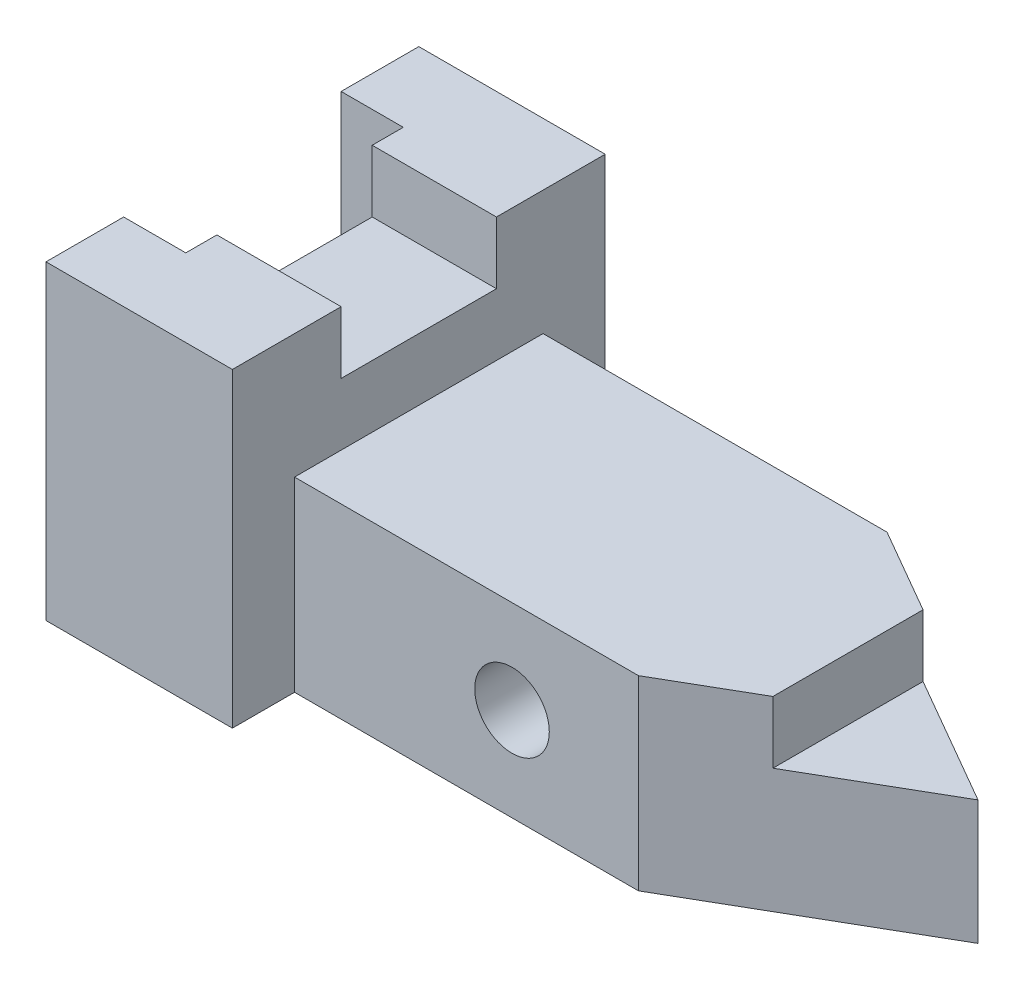
ISO-10303-21;
HEADER;
FILE_DESCRIPTION(('STEP AP214'),'2;1');
FILE_NAME('part.step','',(''),(''),'','','');
FILE_SCHEMA(('AUTOMOTIVE_DESIGN { 1 0 10303 214 1 1 1 1 }'));
ENDSEC;
DATA;
#1=APPLICATION_CONTEXT('core data for automotive mechanical design processes');
#2=APPLICATION_PROTOCOL_DEFINITION('international standard','automotive_design',2000,#1);
#3=PRODUCT_CONTEXT('',#1,'mechanical');
#4=PRODUCT('Part','Part','',(#3));
#5=PRODUCT_RELATED_PRODUCT_CATEGORY('part','',(#4));
#6=PRODUCT_DEFINITION_FORMATION('','',#4);
#7=PRODUCT_DEFINITION_CONTEXT('part definition',#1,'design');
#8=PRODUCT_DEFINITION('design','',#6,#7);
#9=PRODUCT_DEFINITION_SHAPE('','',#8);
#10=(LENGTH_UNIT() NAMED_UNIT(*) SI_UNIT(.MILLI.,.METRE.));
#11=(NAMED_UNIT(*) PLANE_ANGLE_UNIT() SI_UNIT($,.RADIAN.));
#12=(NAMED_UNIT(*) SI_UNIT($,.STERADIAN.) SOLID_ANGLE_UNIT());
#13=UNCERTAINTY_MEASURE_WITH_UNIT(LENGTH_MEASURE(1.E-05),#10,'distance_accuracy_value','');
#14=(GEOMETRIC_REPRESENTATION_CONTEXT(3) GLOBAL_UNCERTAINTY_ASSIGNED_CONTEXT((#13)) GLOBAL_UNIT_ASSIGNED_CONTEXT((#10,
#11,#12)) REPRESENTATION_CONTEXT('',''));
#15=CARTESIAN_POINT('',(0.,0.,0.));
#16=DIRECTION('',(0.,0.,1.));
#17=DIRECTION('',(1.,0.,0.));
#18=AXIS2_PLACEMENT_3D('',#15,#16,#17);
#19=CARTESIAN_POINT('',(0.,0.,30.));
#20=DIRECTION('',(0.,1.,0.));
#21=DIRECTION('',(0.,0.,1.));
#22=AXIS2_PLACEMENT_3D('',#19,#20,#21);
#23=PLANE('',#22);
#24=DIRECTION('',(-1.,0.,0.));
#25=VECTOR('',#24,1.);
#26=CARTESIAN_POINT('',(120.,0.,-20.));
#27=LINE('',#26,#25);
#28=CARTESIAN_POINT('',(85.3589838486219,0.,-20.));
#29=VERTEX_POINT('',#28);
#30=CARTESIAN_POINT('',(30.,0.,-20.));
#31=VERTEX_POINT('',#30);
#32=EDGE_CURVE('E65',#29,#31,#27,.T.);
#33=ORIENTED_EDGE('',*,*,#32,.F.);
#34=DIRECTION('',(-0.866025403784442,0.,-0.499999999999995));
#35=VECTOR('',#34,1.);
#36=CARTESIAN_POINT('',(42.9903810567658,0.,-44.4615242270661));
#37=LINE('',#36,#35);
#38=CARTESIAN_POINT('',(120.,0.,0.));
#39=VERTEX_POINT('',#38);
#40=EDGE_CURVE('E173',#39,#29,#37,.T.);
#41=ORIENTED_EDGE('',*,*,#40,.F.);
#42=DIRECTION('',(-0.866025403784442,0.,0.499999999999995));
#43=VECTOR('',#42,1.);
#44=CARTESIAN_POINT('',(17.0096189432329,0.,59.4615242270658));
#45=LINE('',#44,#43);
#46=CARTESIAN_POINT('',(85.3589838486219,0.,20.));
#47=VERTEX_POINT('',#46);
#48=EDGE_CURVE('E317',#39,#47,#45,.T.);
#49=ORIENTED_EDGE('',*,*,#48,.T.);
#50=DIRECTION('',(-1.,0.,0.));
#51=VECTOR('',#50,1.);
#52=CARTESIAN_POINT('',(120.,0.,20.));
#53=LINE('',#52,#51);
#54=CARTESIAN_POINT('',(30.,0.,20.));
#55=VERTEX_POINT('',#54);
#56=EDGE_CURVE('E194',#47,#55,#53,.T.);
#57=ORIENTED_EDGE('',*,*,#56,.T.);
#58=DIRECTION('',(0.,0.,-1.));
#59=VECTOR('',#58,1.);
#60=CARTESIAN_POINT('',(30.,0.,30.));
#61=LINE('',#60,#59);
#62=CARTESIAN_POINT('',(30.,0.,30.));
#63=VERTEX_POINT('',#62);
#64=EDGE_CURVE('E275',#63,#55,#61,.T.);
#65=ORIENTED_EDGE('',*,*,#64,.F.);
#66=DIRECTION('',(1.,0.,0.));
#67=VECTOR('',#66,1.);
#68=CARTESIAN_POINT('',(0.,0.,30.));
#69=LINE('',#68,#67);
#70=CARTESIAN_POINT('',(0.,0.,30.));
#71=VERTEX_POINT('',#70);
#72=EDGE_CURVE('E247',#71,#63,#69,.T.);
#73=ORIENTED_EDGE('',*,*,#72,.F.);
#74=DIRECTION('',(0.,0.,-1.));
#75=VECTOR('',#74,1.);
#76=CARTESIAN_POINT('',(0.,0.,30.));
#77=LINE('',#76,#75);
#78=CARTESIAN_POINT('',(0.,0.,17.5));
#79=VERTEX_POINT('',#78);
#80=EDGE_CURVE('E277',#71,#79,#77,.T.);
#81=ORIENTED_EDGE('',*,*,#80,.T.);
#82=DIRECTION('',(1.,0.,0.));
#83=VECTOR('',#82,1.);
#84=CARTESIAN_POINT('',(0.,0.,17.5));
#85=LINE('',#84,#83);
#86=CARTESIAN_POINT('',(10.,0.,17.5));
#87=VERTEX_POINT('',#86);
#88=EDGE_CURVE('E230',#79,#87,#85,.T.);
#89=ORIENTED_EDGE('',*,*,#88,.T.);
#90=DIRECTION('',(0.,0.,-1.));
#91=VECTOR('',#90,1.);
#92=CARTESIAN_POINT('',(10.,0.,30.));
#93=LINE('',#92,#91);
#94=CARTESIAN_POINT('',(10.,0.,-17.5));
#95=VERTEX_POINT('',#94);
#96=EDGE_CURVE('E238',#87,#95,#93,.T.);
#97=ORIENTED_EDGE('',*,*,#96,.T.);
#98=DIRECTION('',(-1.,0.,0.));
#99=VECTOR('',#98,1.);
#100=CARTESIAN_POINT('',(0.,0.,-17.5));
#101=LINE('',#100,#99);
#102=CARTESIAN_POINT('',(0.,0.,-17.5));
#103=VERTEX_POINT('',#102);
#104=EDGE_CURVE('E241',#95,#103,#101,.T.);
#105=ORIENTED_EDGE('',*,*,#104,.T.);
#106=CARTESIAN_POINT('',(0.,0.,-30.));
#107=VERTEX_POINT('',#106);
#108=EDGE_CURVE('E273',#103,#107,#77,.T.);
#109=ORIENTED_EDGE('',*,*,#108,.T.);
#110=DIRECTION('',(1.,0.,0.));
#111=VECTOR('',#110,1.);
#112=CARTESIAN_POINT('',(0.,0.,-30.));
#113=LINE('',#112,#111);
#114=CARTESIAN_POINT('',(30.,0.,-30.));
#115=VERTEX_POINT('',#114);
#116=EDGE_CURVE('E259',#107,#115,#113,.T.);
#117=ORIENTED_EDGE('',*,*,#116,.T.);
#118=EDGE_CURVE('E195',#31,#115,#61,.T.);
#119=ORIENTED_EDGE('',*,*,#118,.F.);
#120=EDGE_LOOP('',(#33,#41,#49,#57,#65,#73,#81,#89,#97,#105,#109,#117,#119));
#121=FACE_BOUND('',#120,.T.);
#122=ADVANCED_FACE('F39',(#121),#23,.F.);
#123=CARTESIAN_POINT('',(120.,30.,20.));
#124=DIRECTION('',(0.,-1.,0.));
#125=DIRECTION('',(0.,0.,-1.));
#126=AXIS2_PLACEMENT_3D('',#123,#124,#125);
#127=PLANE('',#126);
#128=DIRECTION('',(-0.866025403784442,0.,-0.499999999999995));
#129=VECTOR('',#128,1.);
#130=CARTESIAN_POINT('',(29.9999999999993,30.,-51.9615242270659));
#131=LINE('',#130,#129);
#132=CARTESIAN_POINT('',(99.0745396778321,30.,-12.0813201499203));
#133=VERTEX_POINT('',#132);
#134=CARTESIAN_POINT('',(85.3589838486219,30.,-20.));
#135=VERTEX_POINT('',#134);
#136=EDGE_CURVE('E325',#133,#135,#131,.T.);
#137=ORIENTED_EDGE('',*,*,#136,.T.);
#138=DIRECTION('',(-1.,0.,0.));
#139=VECTOR('',#138,1.);
#140=CARTESIAN_POINT('',(120.,30.,-20.));
#141=LINE('',#140,#139);
#142=CARTESIAN_POINT('',(30.,30.,-20.));
#143=VERTEX_POINT('',#142);
#144=EDGE_CURVE('E187',#135,#143,#141,.T.);
#145=ORIENTED_EDGE('',*,*,#144,.T.);
#146=DIRECTION('',(0.,0.,1.));
#147=VECTOR('',#146,1.);
#148=CARTESIAN_POINT('',(30.,30.,20.));
#149=LINE('',#148,#147);
#150=CARTESIAN_POINT('',(30.,30.,20.));
#151=VERTEX_POINT('',#150);
#152=EDGE_CURVE('E305',#143,#151,#149,.T.);
#153=ORIENTED_EDGE('',*,*,#152,.T.);
#154=DIRECTION('',(-1.,0.,0.));
#155=VECTOR('',#154,1.);
#156=CARTESIAN_POINT('',(120.,30.,20.));
#157=LINE('',#156,#155);
#158=CARTESIAN_POINT('',(85.3589838486219,30.,20.));
#159=VERTEX_POINT('',#158);
#160=EDGE_CURVE('E53',#159,#151,#157,.T.);
#161=ORIENTED_EDGE('',*,*,#160,.F.);
#162=DIRECTION('',(-0.866025403784442,0.,0.499999999999995));
#163=VECTOR('',#162,1.);
#164=CARTESIAN_POINT('',(29.9999999999994,30.,51.961524227066));
#165=LINE('',#164,#163);
#166=CARTESIAN_POINT('',(99.0745396778321,30.,12.0813201499203));
#167=VERTEX_POINT('',#166);
#168=EDGE_CURVE('E322',#167,#159,#165,.T.);
#169=ORIENTED_EDGE('',*,*,#168,.F.);
#170=DIRECTION('',(0.,0.,1.));
#171=VECTOR('',#170,1.);
#172=CARTESIAN_POINT('',(99.0745396778321,30.,0.));
#173=LINE('',#172,#171);
#174=EDGE_CURVE('E185',#133,#167,#173,.T.);
#175=ORIENTED_EDGE('',*,*,#174,.F.);
#176=EDGE_LOOP('',(#137,#145,#153,#161,#169,#175));
#177=FACE_BOUND('',#176,.T.);
#178=ADVANCED_FACE('F306',(#177),#127,.F.);
#179=CARTESIAN_POINT('',(120.,30.,-20.));
#180=DIRECTION('',(0.,0.,1.));
#181=DIRECTION('',(0.,-1.,0.));
#182=AXIS2_PLACEMENT_3D('',#179,#180,#181);
#183=PLANE('',#182);
#184=CARTESIAN_POINT('',(65.,15.,-20.));
#185=DIRECTION('',(0.,0.,1.));
#186=DIRECTION('',(0.,-1.,0.));
#187=AXIS2_PLACEMENT_3D('',#184,#185,#186);
#188=CIRCLE('',#187,6.);
#189=CARTESIAN_POINT('',(65.,9.,-20.));
#190=VERTEX_POINT('',#189);
#191=EDGE_CURVE('E287',#190,#190,#188,.T.);
#192=ORIENTED_EDGE('',*,*,#191,.T.);
#193=EDGE_LOOP('',(#192));
#194=FACE_BOUND('',#193,.T.);
#195=DIRECTION('',(0.,1.,0.));
#196=VECTOR('',#195,1.);
#197=CARTESIAN_POINT('',(85.3589838486219,0.,-20.));
#198=LINE('',#197,#196);
#199=EDGE_CURVE('E176',#29,#135,#198,.T.);
#200=ORIENTED_EDGE('',*,*,#199,.F.);
#201=ORIENTED_EDGE('',*,*,#32,.T.);
#202=DIRECTION('',(0.,1.,0.));
#203=VECTOR('',#202,1.);
#204=CARTESIAN_POINT('',(30.,30.,-20.));
#205=LINE('',#204,#203);
#206=EDGE_CURVE('E291',#31,#143,#205,.T.);
#207=ORIENTED_EDGE('',*,*,#206,.T.);
#208=ORIENTED_EDGE('',*,*,#144,.F.);
#209=EDGE_LOOP('',(#200,#201,#207,#208));
#210=FACE_BOUND('',#209,.T.);
#211=ADVANCED_FACE('F184',(#194,#210),#183,.F.);
#212=CARTESIAN_POINT('',(99.0745396778321,-30.,0.));
#213=DIRECTION('',(-1.,0.,0.));
#214=DIRECTION('',(0.,0.,1.));
#215=AXIS2_PLACEMENT_3D('',#212,#213,#214);
#216=PLANE('',#215);
#217=DIRECTION('',(0.,1.,0.));
#218=VECTOR('',#217,1.);
#219=CARTESIAN_POINT('',(99.0745396778321,0.,-12.0813201499203));
#220=LINE('',#219,#218);
#221=CARTESIAN_POINT('',(99.0745396778321,20.,-12.0813201499203));
#222=VERTEX_POINT('',#221);
#223=EDGE_CURVE('E189',#222,#133,#220,.T.);
#224=ORIENTED_EDGE('',*,*,#223,.T.);
#225=ORIENTED_EDGE('',*,*,#174,.T.);
#226=DIRECTION('',(0.,1.,0.));
#227=VECTOR('',#226,1.);
#228=CARTESIAN_POINT('',(99.0745396778321,0.,12.0813201499203));
#229=LINE('',#228,#227);
#230=CARTESIAN_POINT('',(99.0745396778321,20.,12.0813201499203));
#231=VERTEX_POINT('',#230);
#232=EDGE_CURVE('E324',#231,#167,#229,.T.);
#233=ORIENTED_EDGE('',*,*,#232,.F.);
#234=DIRECTION('',(0.,0.,1.));
#235=VECTOR('',#234,1.);
#236=CARTESIAN_POINT('',(99.0745396778321,20.,-12.0813201499203));
#237=LINE('',#236,#235);
#238=EDGE_CURVE('E190',#222,#231,#237,.T.);
#239=ORIENTED_EDGE('',*,*,#238,.F.);
#240=EDGE_LOOP('',(#224,#225,#233,#239));
#241=FACE_BOUND('',#240,.T.);
#242=ADVANCED_FACE('F340',(#241),#216,.F.);
#243=CARTESIAN_POINT('',(30.,0.,30.));
#244=DIRECTION('',(-1.,0.,0.));
#245=DIRECTION('',(0.,0.,1.));
#246=AXIS2_PLACEMENT_3D('',#243,#244,#245);
#247=PLANE('',#246);
#248=DIRECTION('',(0.,-1.,0.));
#249=VECTOR('',#248,1.);
#250=CARTESIAN_POINT('',(30.,0.,20.));
#251=LINE('',#250,#249);
#252=EDGE_CURVE('E286',#151,#55,#251,.T.);
#253=ORIENTED_EDGE('',*,*,#252,.F.);
#254=ORIENTED_EDGE('',*,*,#152,.F.);
#255=ORIENTED_EDGE('',*,*,#206,.F.);
#256=ORIENTED_EDGE('',*,*,#118,.T.);
#257=DIRECTION('',(0.,1.,0.));
#258=VECTOR('',#257,1.);
#259=CARTESIAN_POINT('',(30.,0.,-30.));
#260=LINE('',#259,#258);
#261=CARTESIAN_POINT('',(30.,50.,-30.));
#262=VERTEX_POINT('',#261);
#263=EDGE_CURVE('E258',#115,#262,#260,.T.);
#264=ORIENTED_EDGE('',*,*,#263,.T.);
#265=DIRECTION('',(0.,0.,-1.));
#266=VECTOR('',#265,1.);
#267=CARTESIAN_POINT('',(30.,50.,30.));
#268=LINE('',#267,#266);
#269=CARTESIAN_POINT('',(30.,50.,-12.5));
#270=VERTEX_POINT('',#269);
#271=EDGE_CURVE('E267',#270,#262,#268,.T.);
#272=ORIENTED_EDGE('',*,*,#271,.F.);
#273=DIRECTION('',(0.,1.,0.));
#274=VECTOR('',#273,1.);
#275=CARTESIAN_POINT('',(30.,50.,-12.5));
#276=LINE('',#275,#274);
#277=CARTESIAN_POINT('',(30.,40.,-12.5));
#278=VERTEX_POINT('',#277);
#279=EDGE_CURVE('E201',#278,#270,#276,.T.);
#280=ORIENTED_EDGE('',*,*,#279,.F.);
#281=DIRECTION('',(0.,0.,-1.));
#282=VECTOR('',#281,1.);
#283=CARTESIAN_POINT('',(30.,40.,12.5));
#284=LINE('',#283,#282);
#285=CARTESIAN_POINT('',(30.,40.,12.5));
#286=VERTEX_POINT('',#285);
#287=EDGE_CURVE('E204',#286,#278,#284,.T.);
#288=ORIENTED_EDGE('',*,*,#287,.F.);
#289=DIRECTION('',(0.,-1.,0.));
#290=VECTOR('',#289,1.);
#291=CARTESIAN_POINT('',(30.,50.,12.5));
#292=LINE('',#291,#290);
#293=CARTESIAN_POINT('',(30.,50.,12.5));
#294=VERTEX_POINT('',#293);
#295=EDGE_CURVE('E193',#294,#286,#292,.T.);
#296=ORIENTED_EDGE('',*,*,#295,.F.);
#297=CARTESIAN_POINT('',(30.,50.,30.));
#298=VERTEX_POINT('',#297);
#299=EDGE_CURVE('E270',#298,#294,#268,.T.);
#300=ORIENTED_EDGE('',*,*,#299,.F.);
#301=DIRECTION('',(0.,1.,0.));
#302=VECTOR('',#301,1.);
#303=CARTESIAN_POINT('',(30.,0.,30.));
#304=LINE('',#303,#302);
#305=EDGE_CURVE('E252',#63,#298,#304,.T.);
#306=ORIENTED_EDGE('',*,*,#305,.F.);
#307=ORIENTED_EDGE('',*,*,#64,.T.);
#308=EDGE_LOOP('',(#253,#254,#255,#256,#264,#272,#280,#288,#296,#300,#306,#307));
#309=FACE_BOUND('',#308,.T.);
#310=ADVANCED_FACE('F307',(#309),#247,.F.);
#311=CARTESIAN_POINT('',(0.,50.,30.));
#312=DIRECTION('',(0.,-1.,0.));
#313=DIRECTION('',(0.,0.,-1.));
#314=AXIS2_PLACEMENT_3D('',#311,#312,#313);
#315=PLANE('',#314);
#316=ORIENTED_EDGE('',*,*,#299,.T.);
#317=DIRECTION('',(1.,0.,0.));
#318=VECTOR('',#317,1.);
#319=CARTESIAN_POINT('',(-30.,50.,12.5));
#320=LINE('',#319,#318);
#321=CARTESIAN_POINT('',(10.,50.,12.5));
#322=VERTEX_POINT('',#321);
#323=EDGE_CURVE('E206',#322,#294,#320,.T.);
#324=ORIENTED_EDGE('',*,*,#323,.F.);
#325=DIRECTION('',(0.,0.,-1.));
#326=VECTOR('',#325,1.);
#327=CARTESIAN_POINT('',(10.,50.,-17.5));
#328=LINE('',#327,#326);
#329=CARTESIAN_POINT('',(10.,50.,17.5));
#330=VERTEX_POINT('',#329);
#331=EDGE_CURVE('E220',#330,#322,#328,.T.);
#332=ORIENTED_EDGE('',*,*,#331,.F.);
#333=DIRECTION('',(1.,0.,0.));
#334=VECTOR('',#333,1.);
#335=CARTESIAN_POINT('',(0.,50.,17.5));
#336=LINE('',#335,#334);
#337=CARTESIAN_POINT('',(0.,50.,17.5));
#338=VERTEX_POINT('',#337);
#339=EDGE_CURVE('E208',#338,#330,#336,.T.);
#340=ORIENTED_EDGE('',*,*,#339,.F.);
#341=DIRECTION('',(0.,0.,-1.));
#342=VECTOR('',#341,1.);
#343=CARTESIAN_POINT('',(0.,50.,30.));
#344=LINE('',#343,#342);
#345=CARTESIAN_POINT('',(0.,50.,30.));
#346=VERTEX_POINT('',#345);
#347=EDGE_CURVE('E265',#346,#338,#344,.T.);
#348=ORIENTED_EDGE('',*,*,#347,.F.);
#349=DIRECTION('',(-1.,0.,0.));
#350=VECTOR('',#349,1.);
#351=CARTESIAN_POINT('',(0.,50.,30.));
#352=LINE('',#351,#350);
#353=EDGE_CURVE('E254',#298,#346,#352,.T.);
#354=ORIENTED_EDGE('',*,*,#353,.F.);
#355=EDGE_LOOP('',(#316,#324,#332,#340,#348,#354));
#356=FACE_BOUND('',#355,.T.);
#357=ADVANCED_FACE('F358',(#356),#315,.F.);
#358=CARTESIAN_POINT('',(0.,0.,30.));
#359=DIRECTION('',(1.,0.,0.));
#360=DIRECTION('',(0.,0.,-1.));
#361=AXIS2_PLACEMENT_3D('',#358,#359,#360);
#362=PLANE('',#361);
#363=ORIENTED_EDGE('',*,*,#108,.F.);
#364=DIRECTION('',(0.,1.,0.));
#365=VECTOR('',#364,1.);
#366=CARTESIAN_POINT('',(0.,-9.99999999999999,-17.5));
#367=LINE('',#366,#365);
#368=CARTESIAN_POINT('',(0.,50.,-17.5));
#369=VERTEX_POINT('',#368);
#370=EDGE_CURVE('E228',#103,#369,#367,.T.);
#371=ORIENTED_EDGE('',*,*,#370,.T.);
#372=CARTESIAN_POINT('',(0.,50.,-30.));
#373=VERTEX_POINT('',#372);
#374=EDGE_CURVE('E253',#369,#373,#344,.T.);
#375=ORIENTED_EDGE('',*,*,#374,.T.);
#376=DIRECTION('',(0.,-1.,0.));
#377=VECTOR('',#376,1.);
#378=CARTESIAN_POINT('',(0.,0.,-30.));
#379=LINE('',#378,#377);
#380=EDGE_CURVE('E242',#373,#107,#379,.T.);
#381=ORIENTED_EDGE('',*,*,#380,.T.);
#382=EDGE_LOOP('',(#363,#371,#375,#381));
#383=FACE_BOUND('',#382,.T.);
#384=ADVANCED_FACE('F502',(#383),#362,.F.);
#385=ORIENTED_EDGE('',*,*,#347,.T.);
#386=DIRECTION('',(0.,1.,0.));
#387=VECTOR('',#386,1.);
#388=CARTESIAN_POINT('',(0.,-9.99999999999999,17.5));
#389=LINE('',#388,#387);
#390=EDGE_CURVE('E221',#79,#338,#389,.T.);
#391=ORIENTED_EDGE('',*,*,#390,.F.);
#392=ORIENTED_EDGE('',*,*,#80,.F.);
#393=DIRECTION('',(0.,-1.,0.));
#394=VECTOR('',#393,1.);
#395=CARTESIAN_POINT('',(0.,0.,30.));
#396=LINE('',#395,#394);
#397=EDGE_CURVE('E244',#346,#71,#396,.T.);
#398=ORIENTED_EDGE('',*,*,#397,.F.);
#399=EDGE_LOOP('',(#385,#391,#392,#398));
#400=FACE_BOUND('',#399,.T.);
#401=ADVANCED_FACE('F41',(#400),#362,.F.);
#402=CARTESIAN_POINT('',(10.,50.,-12.5));
#403=VERTEX_POINT('',#402);
#404=CARTESIAN_POINT('',(10.,50.,-17.5));
#405=VERTEX_POINT('',#404);
#406=EDGE_CURVE('E218',#403,#405,#328,.T.);
#407=ORIENTED_EDGE('',*,*,#406,.F.);
#408=DIRECTION('',(1.,0.,0.));
#409=VECTOR('',#408,1.);
#410=CARTESIAN_POINT('',(-30.,50.,-12.5));
#411=LINE('',#410,#409);
#412=EDGE_CURVE('E212',#403,#270,#411,.T.);
#413=ORIENTED_EDGE('',*,*,#412,.T.);
#414=ORIENTED_EDGE('',*,*,#271,.T.);
#415=DIRECTION('',(-1.,0.,0.));
#416=VECTOR('',#415,1.);
#417=CARTESIAN_POINT('',(0.,50.,-30.));
#418=LINE('',#417,#416);
#419=EDGE_CURVE('E248',#262,#373,#418,.T.);
#420=ORIENTED_EDGE('',*,*,#419,.T.);
#421=ORIENTED_EDGE('',*,*,#374,.F.);
#422=DIRECTION('',(-1.,0.,0.));
#423=VECTOR('',#422,1.);
#424=CARTESIAN_POINT('',(0.,50.,-17.5));
#425=LINE('',#424,#423);
#426=EDGE_CURVE('E222',#405,#369,#425,.T.);
#427=ORIENTED_EDGE('',*,*,#426,.F.);
#428=EDGE_LOOP('',(#407,#413,#414,#420,#421,#427));
#429=FACE_BOUND('',#428,.T.);
#430=ADVANCED_FACE('F357',(#429),#315,.F.);
#431=CARTESIAN_POINT('',(0.,0.,30.));
#432=DIRECTION('',(0.,0.,-1.));
#433=DIRECTION('',(-1.,0.,0.));
#434=AXIS2_PLACEMENT_3D('',#431,#432,#433);
#435=PLANE('',#434);
#436=ORIENTED_EDGE('',*,*,#397,.T.);
#437=ORIENTED_EDGE('',*,*,#72,.T.);
#438=ORIENTED_EDGE('',*,*,#305,.T.);
#439=ORIENTED_EDGE('',*,*,#353,.T.);
#440=EDGE_LOOP('',(#436,#437,#438,#439));
#441=FACE_BOUND('',#440,.T.);
#442=ADVANCED_FACE('F359',(#441),#435,.F.);
#443=CARTESIAN_POINT('',(0.,0.,-30.));
#444=DIRECTION('',(0.,0.,-1.));
#445=DIRECTION('',(-1.,0.,0.));
#446=AXIS2_PLACEMENT_3D('',#443,#444,#445);
#447=PLANE('',#446);
#448=ORIENTED_EDGE('',*,*,#380,.F.);
#449=ORIENTED_EDGE('',*,*,#419,.F.);
#450=ORIENTED_EDGE('',*,*,#263,.F.);
#451=ORIENTED_EDGE('',*,*,#116,.F.);
#452=EDGE_LOOP('',(#448,#449,#450,#451));
#453=FACE_BOUND('',#452,.T.);
#454=ADVANCED_FACE('F365',(#453),#447,.T.);
#455=CARTESIAN_POINT('',(0.,-9.99999999999999,-17.5));
#456=DIRECTION('',(0.,0.,-1.));
#457=DIRECTION('',(-1.,0.,0.));
#458=AXIS2_PLACEMENT_3D('',#455,#456,#457);
#459=PLANE('',#458);
#460=DIRECTION('',(0.,1.,0.));
#461=VECTOR('',#460,1.);
#462=CARTESIAN_POINT('',(10.,-9.99999999999999,-17.5));
#463=LINE('',#462,#461);
#464=EDGE_CURVE('E229',#95,#405,#463,.T.);
#465=ORIENTED_EDGE('',*,*,#464,.T.);
#466=ORIENTED_EDGE('',*,*,#426,.T.);
#467=ORIENTED_EDGE('',*,*,#370,.F.);
#468=ORIENTED_EDGE('',*,*,#104,.F.);
#469=EDGE_LOOP('',(#465,#466,#467,#468));
#470=FACE_BOUND('',#469,.T.);
#471=ADVANCED_FACE('F362',(#470),#459,.F.);
#472=CARTESIAN_POINT('',(10.,-9.99999999999999,-17.5));
#473=DIRECTION('',(1.,0.,0.));
#474=DIRECTION('',(0.,0.,-1.));
#475=AXIS2_PLACEMENT_3D('',#472,#473,#474);
#476=PLANE('',#475);
#477=ORIENTED_EDGE('',*,*,#331,.T.);
#478=DIRECTION('',(0.,-1.,0.));
#479=VECTOR('',#478,1.);
#480=CARTESIAN_POINT('',(10.,-10.,12.5));
#481=LINE('',#480,#479);
#482=CARTESIAN_POINT('',(10.,40.,12.5));
#483=VERTEX_POINT('',#482);
#484=EDGE_CURVE('E285',#322,#483,#481,.T.);
#485=ORIENTED_EDGE('',*,*,#484,.T.);
#486=DIRECTION('',(0.,0.,-1.));
#487=VECTOR('',#486,1.);
#488=CARTESIAN_POINT('',(10.,40.,-17.5));
#489=LINE('',#488,#487);
#490=CARTESIAN_POINT('',(10.,40.,-12.5));
#491=VERTEX_POINT('',#490);
#492=EDGE_CURVE('E276',#483,#491,#489,.T.);
#493=ORIENTED_EDGE('',*,*,#492,.T.);
#494=DIRECTION('',(0.,1.,0.));
#495=VECTOR('',#494,1.);
#496=CARTESIAN_POINT('',(10.,-10.,-12.5));
#497=LINE('',#496,#495);
#498=EDGE_CURVE('E282',#491,#403,#497,.T.);
#499=ORIENTED_EDGE('',*,*,#498,.T.);
#500=ORIENTED_EDGE('',*,*,#406,.T.);
#501=ORIENTED_EDGE('',*,*,#464,.F.);
#502=ORIENTED_EDGE('',*,*,#96,.F.);
#503=DIRECTION('',(0.,1.,0.));
#504=VECTOR('',#503,1.);
#505=CARTESIAN_POINT('',(10.,-9.99999999999999,17.5));
#506=LINE('',#505,#504);
#507=EDGE_CURVE('E231',#87,#330,#506,.T.);
#508=ORIENTED_EDGE('',*,*,#507,.T.);
#509=EDGE_LOOP('',(#477,#485,#493,#499,#500,#501,#502,#508));
#510=FACE_BOUND('',#509,.T.);
#511=ADVANCED_FACE('F372',(#510),#476,.F.);
#512=CARTESIAN_POINT('',(0.,-9.99999999999999,17.5));
#513=DIRECTION('',(0.,0.,1.));
#514=DIRECTION('',(1.,0.,0.));
#515=AXIS2_PLACEMENT_3D('',#512,#513,#514);
#516=PLANE('',#515);
#517=ORIENTED_EDGE('',*,*,#390,.T.);
#518=ORIENTED_EDGE('',*,*,#339,.T.);
#519=ORIENTED_EDGE('',*,*,#507,.F.);
#520=ORIENTED_EDGE('',*,*,#88,.F.);
#521=EDGE_LOOP('',(#517,#518,#519,#520));
#522=FACE_BOUND('',#521,.T.);
#523=ADVANCED_FACE('F369',(#522),#516,.F.);
#524=CARTESIAN_POINT('',(-30.,50.,12.5));
#525=DIRECTION('',(0.,0.,1.));
#526=DIRECTION('',(0.,-1.,0.));
#527=AXIS2_PLACEMENT_3D('',#524,#525,#526);
#528=PLANE('',#527);
#529=ORIENTED_EDGE('',*,*,#323,.T.);
#530=ORIENTED_EDGE('',*,*,#295,.T.);
#531=DIRECTION('',(1.,0.,0.));
#532=VECTOR('',#531,1.);
#533=CARTESIAN_POINT('',(-30.,40.,12.5));
#534=LINE('',#533,#532);
#535=EDGE_CURVE('E210',#483,#286,#534,.T.);
#536=ORIENTED_EDGE('',*,*,#535,.F.);
#537=ORIENTED_EDGE('',*,*,#484,.F.);
#538=EDGE_LOOP('',(#529,#530,#536,#537));
#539=FACE_BOUND('',#538,.T.);
#540=ADVANCED_FACE('F373',(#539),#528,.F.);
#541=CARTESIAN_POINT('',(-30.,50.,-12.5));
#542=DIRECTION('',(0.,0.,-1.));
#543=DIRECTION('',(0.,1.,0.));
#544=AXIS2_PLACEMENT_3D('',#541,#542,#543);
#545=PLANE('',#544);
#546=DIRECTION('',(1.,0.,0.));
#547=VECTOR('',#546,1.);
#548=CARTESIAN_POINT('',(-30.,40.,-12.5));
#549=LINE('',#548,#547);
#550=EDGE_CURVE('E211',#491,#278,#549,.T.);
#551=ORIENTED_EDGE('',*,*,#550,.T.);
#552=ORIENTED_EDGE('',*,*,#279,.T.);
#553=ORIENTED_EDGE('',*,*,#412,.F.);
#554=ORIENTED_EDGE('',*,*,#498,.F.);
#555=EDGE_LOOP('',(#551,#552,#553,#554));
#556=FACE_BOUND('',#555,.T.);
#557=ADVANCED_FACE('F381',(#556),#545,.F.);
#558=CARTESIAN_POINT('',(-30.,40.,12.5));
#559=DIRECTION('',(0.,-1.,0.));
#560=DIRECTION('',(0.,0.,-1.));
#561=AXIS2_PLACEMENT_3D('',#558,#559,#560);
#562=PLANE('',#561);
#563=ORIENTED_EDGE('',*,*,#535,.T.);
#564=ORIENTED_EDGE('',*,*,#287,.T.);
#565=ORIENTED_EDGE('',*,*,#550,.F.);
#566=ORIENTED_EDGE('',*,*,#492,.F.);
#567=EDGE_LOOP('',(#563,#564,#565,#566));
#568=FACE_BOUND('',#567,.T.);
#569=ADVANCED_FACE('F387',(#568),#562,.F.);
#570=CARTESIAN_POINT('',(120.,0.,20.));
#571=DIRECTION('',(0.,0.,-1.));
#572=DIRECTION('',(-1.,0.,0.));
#573=AXIS2_PLACEMENT_3D('',#570,#571,#572);
#574=PLANE('',#573);
#575=CARTESIAN_POINT('',(65.,15.,20.));
#576=DIRECTION('',(0.,0.,1.));
#577=DIRECTION('',(1.,0.,0.));
#578=AXIS2_PLACEMENT_3D('',#575,#576,#577);
#579=CIRCLE('',#578,6.);
#580=CARTESIAN_POINT('',(71.,15.,20.));
#581=VERTEX_POINT('',#580);
#582=EDGE_CURVE('E181',#581,#581,#579,.T.);
#583=ORIENTED_EDGE('',*,*,#582,.F.);
#584=EDGE_LOOP('',(#583));
#585=FACE_BOUND('',#584,.T.);
#586=ORIENTED_EDGE('',*,*,#56,.F.);
#587=DIRECTION('',(0.,1.,0.));
#588=VECTOR('',#587,1.);
#589=CARTESIAN_POINT('',(85.3589838486219,0.,20.));
#590=LINE('',#589,#588);
#591=EDGE_CURVE('E314',#47,#159,#590,.T.);
#592=ORIENTED_EDGE('',*,*,#591,.T.);
#593=ORIENTED_EDGE('',*,*,#160,.T.);
#594=ORIENTED_EDGE('',*,*,#252,.T.);
#595=EDGE_LOOP('',(#586,#592,#593,#594));
#596=FACE_BOUND('',#595,.T.);
#597=ADVANCED_FACE('F312',(#585,#596),#574,.F.);
#598=CARTESIAN_POINT('',(65.,15.,-40.));
#599=DIRECTION('',(0.,0.,1.));
#600=DIRECTION('',(1.,0.,0.));
#601=AXIS2_PLACEMENT_3D('',#598,#599,#600);
#602=CYLINDRICAL_SURFACE('',#601,6.);
#603=ORIENTED_EDGE('',*,*,#582,.T.);
#604=EDGE_LOOP('',(#603));
#605=FACE_BOUND('',#604,.T.);
#606=ORIENTED_EDGE('',*,*,#191,.F.);
#607=EDGE_LOOP('',(#606));
#608=FACE_BOUND('',#607,.T.);
#609=ADVANCED_FACE('F395',(#605,#608),#602,.F.);
#610=CARTESIAN_POINT('',(29.9999999999993,-30.,-51.9615242270659));
#611=DIRECTION('',(0.499999999999994,0.,-0.866025403784442));
#612=DIRECTION('',(-0.866025403784442,0.,-0.499999999999995));
#613=AXIS2_PLACEMENT_3D('',#610,#611,#612);
#614=PLANE('',#613);
#615=DIRECTION('',(-0.866025403784442,0.,-0.499999999999995));
#616=VECTOR('',#615,1.);
#617=CARTESIAN_POINT('',(29.9999999999993,20.,-51.9615242270659));
#618=LINE('',#617,#616);
#619=CARTESIAN_POINT('',(120.,20.,0.));
#620=VERTEX_POINT('',#619);
#621=EDGE_CURVE('E319',#620,#222,#618,.T.);
#622=ORIENTED_EDGE('',*,*,#621,.F.);
#623=DIRECTION('',(0.,-1.,0.));
#624=VECTOR('',#623,1.);
#625=CARTESIAN_POINT('',(120.,0.,0.));
#626=LINE('',#625,#624);
#627=EDGE_CURVE('E50',#620,#39,#626,.T.);
#628=ORIENTED_EDGE('',*,*,#627,.T.);
#629=ORIENTED_EDGE('',*,*,#40,.T.);
#630=ORIENTED_EDGE('',*,*,#199,.T.);
#631=ORIENTED_EDGE('',*,*,#136,.F.);
#632=ORIENTED_EDGE('',*,*,#223,.F.);
#633=EDGE_LOOP('',(#622,#628,#629,#630,#631,#632));
#634=FACE_BOUND('',#633,.T.);
#635=ADVANCED_FACE('F174',(#634),#614,.T.);
#636=CARTESIAN_POINT('',(29.9999999999994,-30.,51.961524227066));
#637=DIRECTION('',(-0.499999999999995,0.,-0.866025403784442));
#638=DIRECTION('',(-0.866025403784442,0.,0.499999999999995));
#639=AXIS2_PLACEMENT_3D('',#636,#637,#638);
#640=PLANE('',#639);
#641=ORIENTED_EDGE('',*,*,#627,.F.);
#642=DIRECTION('',(-0.866025403784442,0.,0.499999999999995));
#643=VECTOR('',#642,1.);
#644=CARTESIAN_POINT('',(29.9999999999994,20.,51.961524227066));
#645=LINE('',#644,#643);
#646=EDGE_CURVE('E11',#620,#231,#645,.T.);
#647=ORIENTED_EDGE('',*,*,#646,.T.);
#648=ORIENTED_EDGE('',*,*,#232,.T.);
#649=ORIENTED_EDGE('',*,*,#168,.T.);
#650=ORIENTED_EDGE('',*,*,#591,.F.);
#651=ORIENTED_EDGE('',*,*,#48,.F.);
#652=EDGE_LOOP('',(#641,#647,#648,#649,#650,#651));
#653=FACE_BOUND('',#652,.T.);
#654=ADVANCED_FACE('F318',(#653),#640,.F.);
#655=CARTESIAN_POINT('',(0.,20.,0.));
#656=DIRECTION('',(0.,-1.,0.));
#657=DIRECTION('',(0.,0.,-1.));
#658=AXIS2_PLACEMENT_3D('',#655,#656,#657);
#659=PLANE('',#658);
#660=ORIENTED_EDGE('',*,*,#621,.T.);
#661=ORIENTED_EDGE('',*,*,#238,.T.);
#662=ORIENTED_EDGE('',*,*,#646,.F.);
#663=EDGE_LOOP('',(#660,#661,#662));
#664=FACE_BOUND('',#663,.T.);
#665=ADVANCED_FACE('F338',(#664),#659,.F.);
#666=CLOSED_SHELL('',(#122,#178,#211,#242,#310,#357,#384,#401,#430,#442,#454,#471,#511,#523,
#540,#557,#569,#597,#609,#635,#654,#665));
#667=MANIFOLD_SOLID_BREP('B2',#666);
#668=ADVANCED_BREP_SHAPE_REPRESENTATION('',(#18,#667),#14);
#669=SHAPE_DEFINITION_REPRESENTATION(#9,#668);
ENDSEC;
END-ISO-10303-21;
